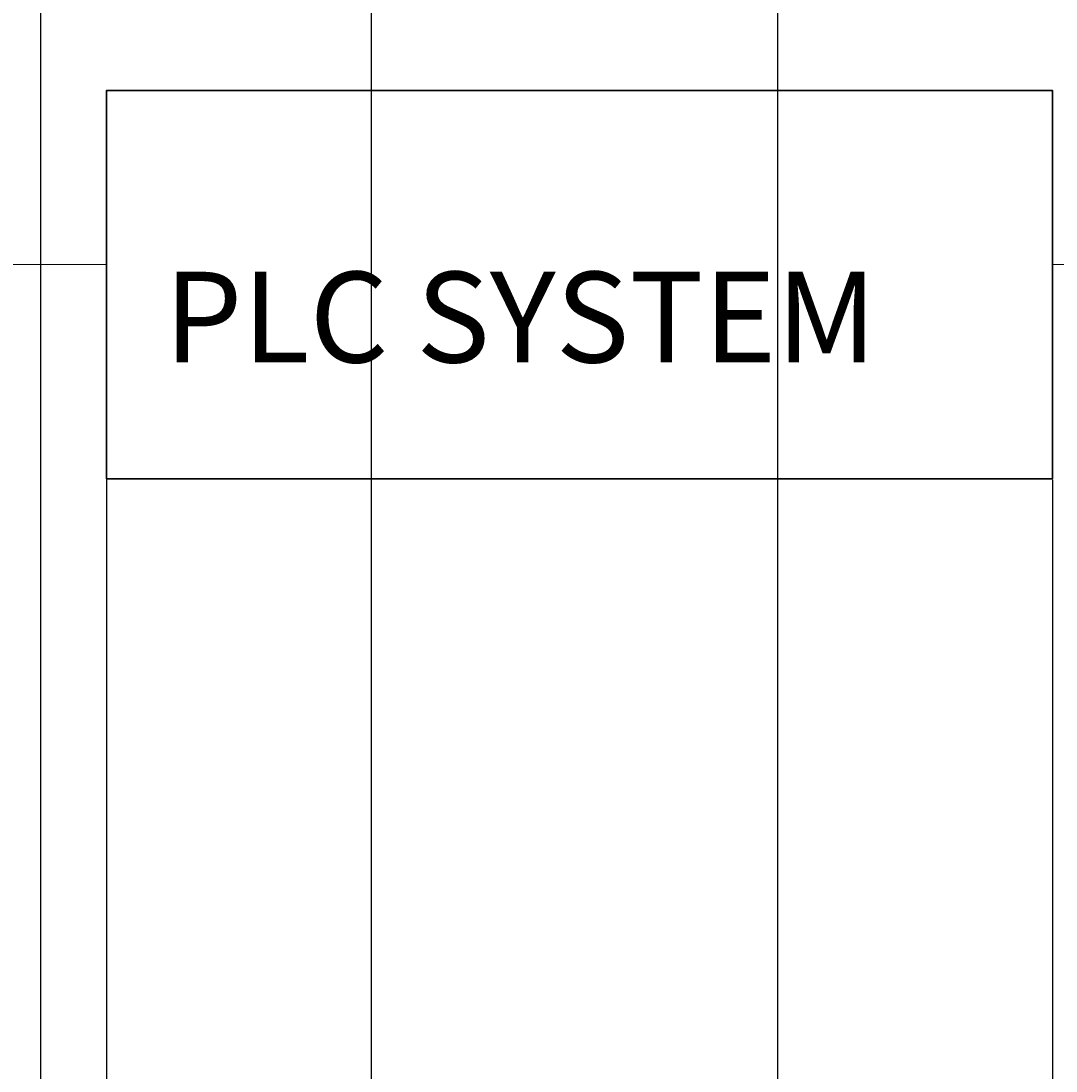
# Model space of a CAD drawing. Units: inches. Extents: x 738 to 1068, y 378 to 757.
# Tile 31 of 41: x 882 to 939, y 549 to 606. Entities that reach past the tile are written whole.
import ezdxf

# ---------------------------------------------------------------- set-up
doc = ezdxf.new("R2010")
doc.units = ezdxf.units.IN
doc.header["$MEASUREMENT"] = 0
for name, color, linetype, lineweight in [('A-ANNO-DIMS', 2, 'Continuous', 18), ('E-ANNO-TEXT', 7, 'Continuous', 18), ('E-CTRL-EQPM', 4, 'Continuous', 35), ('E-CTRL-WIRE', 7, 'Continuous', 18)]:
    doc.layers.add(name, color=color, linetype=linetype, lineweight=lineweight)
doc.styles.get("Standard").update_dxf_attribs({"font": 'arial.ttf'})
doc.dimstyles.get("Standard").update_dxf_attribs({"dimtxt": 0.18, "dimasz": 0.18, "dimexe": 0.18, "dimexo": 0.0625, "dimgap": 0.09, "dimtad": 0, "dimtih": 1, "dimtoh": 1, "dimdec": 4, "dimzin": 0, "dimdsep": 46, "dimtxsty": 'Standard', "dimcen": 0.09, "dimadec": 0, "dimazin": 0, "dimtfac": 1, "dimtdec": 4, "dimtofl": 0, "dimtmove": 0, "dimatfit": 3, "dimfxl": 1, "dimtolj": 1, "dimtzin": 0, "dimarcsym": 0})

# ---------------------------------------------------------------- blocks, each defined once
blk = doc.blocks.new('*D18')
at = {"layer": 'A-ANNO-DIMS', "color": 0, "lineweight": -2, "transparency": 16777216}
for p, q in [((901.525, 738.375), (1068.179, 738.375)), ((1067.999, 738.195), (1067.999, 569.167)), ((1067.999, 399.775), (1067.999, 568.803)), ((1023.842, 399.595), (1068.179, 399.595))]:
    blk.add_line(p, q, dxfattribs=at)
at = {"layer": 'A-ANNO-DIMS', "color": 0, "transparency": 16777216}
for points in [[(1067.969, 738.195), (1068.029, 738.195), (1067.999, 738.375)], [(1067.969, 399.775), (1068.029, 399.775), (1067.999, 399.595)]]:
    blk.add_solid(points, dxfattribs=at)
at = {"layer": 'Defpoints', "color": 0, "transparency": 16777216}
for p in [(901.462, 738.375), (1067.999, 738.375), (1023.779, 399.595)]:
    blk.add_point(p, dxfattribs=at)
at = {"layer": 'A-ANNO-DIMS', "color": 0, "transparency": 16777216, "insert": (1067.999, 568.985), "char_height": 0.18, "attachment_point": 5}
blk.add_mtext('\\A1;338.8', dxfattribs=at)
blk = doc.blocks.new('*D27')
at = {"layer": 'A-ANNO-DIMS', "color": 0, "lineweight": -2, "transparency": 16777216}
for p, q in [((883.457, 646.923), (883.457, 378.239)), ((923.511, 646.923), (923.511, 378.239)), ((883.637, 378.419), (903.086, 378.419)), ((923.331, 378.419), (903.882, 378.419))]:
    blk.add_line(p, q, dxfattribs=at)
at = {"layer": 'A-ANNO-DIMS', "color": 0, "transparency": 16777216}
for points in [[(883.637, 378.449), (883.637, 378.389), (883.457, 378.419)], [(923.331, 378.449), (923.331, 378.389), (923.511, 378.419)]]:
    blk.add_solid(points, dxfattribs=at)
at = {"layer": 'Defpoints', "color": 0, "transparency": 16777216}
for p in [(883.457, 646.985), (923.511, 646.985), (923.511, 378.419)]:
    blk.add_point(p, dxfattribs=at)
at = {"layer": 'A-ANNO-DIMS', "color": 0, "transparency": 16777216, "insert": (903.484, 378.419), "char_height": 0.18, "attachment_point": 5}
blk.add_mtext('\\A1;40.05', dxfattribs=at)
blk = doc.blocks.new('*D28')
at = {"layer": 'A-ANNO-DIMS', "color": 0, "lineweight": -2, "transparency": 16777216}
for p, q in [((923.511, 646.923), (923.511, 378.239)), ((969.439, 646.923), (969.439, 378.239)), ((923.691, 378.419), (946.078, 378.419)), ((969.259, 378.419), (946.872, 378.419))]:
    blk.add_line(p, q, dxfattribs=at)
at = {"layer": 'A-ANNO-DIMS', "color": 0, "transparency": 16777216}
for points in [[(923.691, 378.449), (923.691, 378.389), (923.511, 378.419)], [(969.259, 378.449), (969.259, 378.389), (969.439, 378.419)]]:
    blk.add_solid(points, dxfattribs=at)
at = {"layer": 'Defpoints', "color": 0, "transparency": 16777216}
for p in [(923.511, 646.985), (969.439, 646.985), (969.439, 378.419)]:
    blk.add_point(p, dxfattribs=at)
at = {"layer": 'A-ANNO-DIMS', "color": 0, "transparency": 16777216, "insert": (946.475, 378.419), "char_height": 0.18, "attachment_point": 5}
blk.add_mtext('\\A1;45.93', dxfattribs=at)
blk = doc.blocks.new('*D35')
at = {"layer": 'A-ANNO-DIMS', "color": 0, "lineweight": -2, "transparency": 16777216}
for p, q in [((855.932, 686.266), (855.932, 378.239)), ((901.429, 686.267), (901.429, 378.239)), ((856.112, 378.419), (878.352, 378.419)), ((901.249, 378.419), (879.009, 378.419))]:
    blk.add_line(p, q, dxfattribs=at)
at = {"layer": 'A-ANNO-DIMS', "color": 0, "transparency": 16777216}
for points in [[(856.112, 378.449), (856.112, 378.389), (855.932, 378.419)], [(901.249, 378.449), (901.249, 378.389), (901.429, 378.419)]]:
    blk.add_solid(points, dxfattribs=at)
at = {"layer": 'Defpoints', "color": 0, "transparency": 16777216}
for p in [(855.932, 686.329), (901.429, 686.329), (901.429, 378.419)]:
    blk.add_point(p, dxfattribs=at)
at = {"layer": 'A-ANNO-DIMS', "color": 0, "transparency": 16777216, "insert": (878.68, 378.419), "char_height": 0.18, "attachment_point": 5}
blk.add_mtext('\\A1;45.5', dxfattribs=at)
blk = doc.blocks.new('*D38')
at = {"layer": 'A-ANNO-DIMS', "color": 0, "lineweight": -2, "transparency": 16777216}
for p, q in [((781.485, 593.017), (781.485, 378.239)), ((887.04, 593.067), (887.04, 378.239)), ((781.665, 378.419), (833.807, 378.419)), ((886.86, 378.419), (834.718, 378.419))]:
    blk.add_line(p, q, dxfattribs=at)
at = {"layer": 'A-ANNO-DIMS', "color": 0, "transparency": 16777216}
for points in [[(781.665, 378.449), (781.665, 378.389), (781.485, 378.419)], [(886.86, 378.449), (886.86, 378.389), (887.04, 378.419)]]:
    blk.add_solid(points, dxfattribs=at)
at = {"layer": 'Defpoints', "color": 0, "transparency": 16777216}
for p in [(781.485, 593.08), (887.04, 593.13), (887.04, 378.419)]:
    blk.add_point(p, dxfattribs=at)
at = {"layer": 'A-ANNO-DIMS', "color": 0, "transparency": 16777216, "insert": (834.263, 378.419), "char_height": 0.18, "attachment_point": 5}
blk.add_mtext('\\A1;105.56', dxfattribs=at)
blk = doc.blocks.new('*D39')
at = {"layer": 'A-ANNO-DIMS', "color": 0, "lineweight": -2, "transparency": 16777216}
for p, q in [((887.04, 581.418), (887.04, 378.239)), ((938.455, 581.418), (938.455, 378.239)), ((887.22, 378.419), (912.371, 378.419)), ((938.275, 378.419), (913.124, 378.419))]:
    blk.add_line(p, q, dxfattribs=at)
at = {"layer": 'A-ANNO-DIMS', "color": 0, "transparency": 16777216}
for points in [[(887.22, 378.449), (887.22, 378.389), (887.04, 378.419)], [(938.275, 378.449), (938.275, 378.389), (938.455, 378.419)]]:
    blk.add_solid(points, dxfattribs=at)
at = {"layer": 'Defpoints', "color": 0, "transparency": 16777216}
for p in [(887.04, 581.481), (938.455, 581.481), (938.455, 378.419)]:
    blk.add_point(p, dxfattribs=at)
at = {"layer": 'A-ANNO-DIMS', "color": 0, "transparency": 16777216, "insert": (912.748, 378.419), "char_height": 0.18, "attachment_point": 5}
blk.add_mtext('\\A1;51.41', dxfattribs=at)

msp = doc.modelspace()

# ---------------------------------------------------------------- linework, layer by layer
at = {"layer": 'E-CTRL-EQPM'}
msp.add_lwpolyline([(887.0404, 581.4808), (938.455, 581.4808), (938.455, 602.5631), (887.0404, 602.5631)], close=True, dxfattribs=at)
at = {"layer": 'E-CTRL-WIRE'}
for p, q in [((781.4897, 593.1296), (887.0404, 593.1296)), ((938.455, 593.1296), (1023.824, 593.1296))]:
    msp.add_line(p, q, dxfattribs=at)

# ---------------------------------------------------------------- texts
at = {"layer": 'E-ANNO-TEXT'}
msp.add_text('PLC SYSTEM', height=4.92799, dxfattribs=at).set_placement((890.171, 587.799))

# ---------------------------------------------------------------- dimensions: what is measured, and where the dimension line sits
at = {"layer": 'A-ANNO-DIMS'}
dim = msp.add_linear_dim(base=(1067.9992, 738.3751), p1=(1023.779, 399.5952), p2=(901.4622, 738.3751), angle=90, dimstyle='Standard', override={"dimdec": 1, "dimlfac": 1, "dimrnd": 0, "dimzin": 0, "dimdsep": 46, "dimlunit": 2}, dxfattribs=at)
dim.commit()
dim.dimension.update_dxf_attribs({"geometry": '*D18', "text_midpoint": (1067.9992, 568.9851)})
for base, p1, p2, override, picture, middle in [((901.4286, 378.4191), (855.9323, 686.329), (901.4286, 686.3292), {"dimdec": 1, "dimlfac": 1, "dimrnd": 0, "dimzin": 0, "dimdsep": 46, "dimlunit": 2}, '*D35', (878.6804, 378.4191)), ((923.5105, 378.4191), (883.4574, 646.9853), (923.5105, 646.9853), {"dimdec": 2, "dimlfac": 1, "dimrnd": 0, "dimzin": 0, "dimdsep": 46, "dimlunit": 2}, '*D27', (903.484, 378.4191)), ((969.4395, 378.4191), (923.5105, 646.9853), (969.4395, 646.9853), {"dimdec": 2, "dimlfac": 1, "dimrnd": 0, "dimzin": 0, "dimdsep": 46, "dimlunit": 2}, '*D28', (946.475, 378.4191)), ((887.0404, 378.4191), (781.4846, 593.0796), (887.0404, 593.1296), {"dimdec": 2, "dimlfac": 1, "dimrnd": 0, "dimzin": 0, "dimdsep": 46, "dimlunit": 2}, '*D38', (834.2625, 378.4191)), ((938.455, 378.4191), (887.0404, 581.4808), (938.455, 581.4808), {"dimdec": 2, "dimlfac": 1, "dimrnd": 0, "dimzin": 0, "dimdsep": 46, "dimlunit": 2}, '*D39', (912.7477, 378.4191))]:
    dim = msp.add_linear_dim(base=base, p1=p1, p2=p2, dimstyle='Standard', override=override, dxfattribs=at)
    dim.commit()
    dim.dimension.update_dxf_attribs({"geometry": picture, "text_midpoint": middle})

doc.saveas('drawing.dxf')
